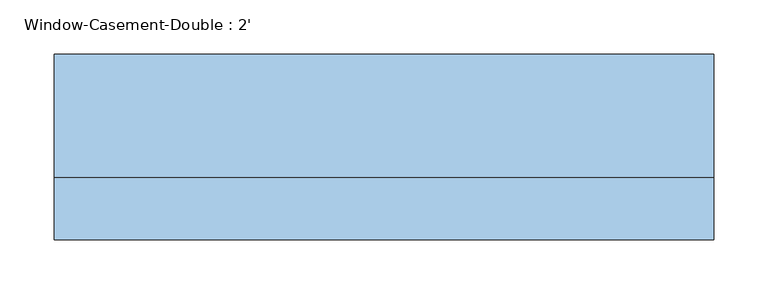
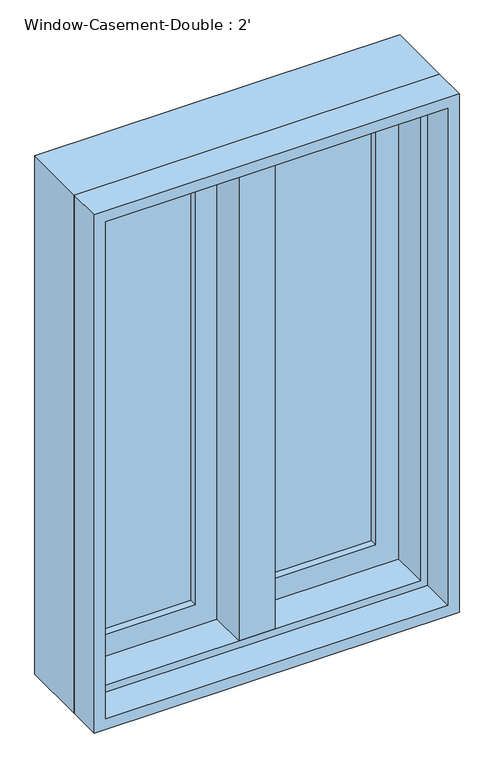
"""IFC4 building model written with IfcOpenShell, lengths in millimetres: window geometry, Window-Casement-Double : 2'."""

from ifc_helpers import new_model, si_unit, frame, origin, place, context, project, spatial, polyline, outline, extrude, faceted_brep, source, transform, mapped, element, save


def window_casement_double_2_fb285ced(model_context):
    return source(origin(), model_context, "Body", "SolidModel", [
        faceted_brep([(9.525, 95.25, 1816.1), (-9.525, 95.25, 1816.1), (-9.525, 44.45, 1816.1), (9.525, 44.45, 1816.1), (9.525, 95.25, 927.1), (9.525, 44.45, 927.1), (-9.525, 44.45, 927.1), (-9.525, 95.25, 927.1), (-9.525, 44.45, 946.15), (-9.525, 44.45, 1797.05), (-30.1625, 44.45, 946.15), (-30.1625, 44.45, 1797.05), (-30.1625, -19.05, 946.15), (-30.1625, -19.05, 1797.05), (30.1625, -19.05, 946.15), (30.1625, -19.05, 1797.05), (30.1625, 44.45, 946.15), (30.1625, 44.45, 1797.05), (9.525, 44.45, 946.15), (9.525, 44.45, 1797.05)], [[[0, 1, 2, 3]], [[4, 5, 6, 7]], [[1, 0, 4, 7]], [[2, 1, 7, 6, 8, 9]], [[9, 8, 10, 11]], [[11, 10, 12, 13]], [[13, 12, 14, 15]], [[15, 14, 16, 17]], [[17, 16, 18, 19]], [[0, 3, 19, 18, 5, 4]], [[18, 8, 6, 5]], [[9, 19, 3, 2]], [[8, 18, 16, 14, 12, 10]], [[19, 9, 11, 13, 15, 17]]]),
        extrude(outline(polyline([(-66.675, 76.2), (-66.675, 69.85), (-234.95, 69.85), (-234.95, 76.2), (-66.675, 76.2)])), frame((0.0, 0.0, 984.25), z_axis=(0.0, 0.0, 1.0), x_axis=(1.0, 0.0, 0.0)), (0.0, 0.0, 1.0), 774.7),
        extrude(outline(polyline([(-234.95, 57.15), (-234.95, 63.5), (-66.675, 63.5), (-66.675, 57.15), (-234.95, 57.15)])), frame((0.0, 0.0, 984.25), z_axis=(0.0, 0.0, 1.0), x_axis=(1.0, 0.0, 0.0)), (0.0, 0.0, 1.0), 774.7),
        extrude(outline(polyline([(234.95, 76.2), (234.95, 69.85), (66.675, 69.85), (66.675, 76.2), (234.95, 76.2)])), frame((0.0, 0.0, 984.25), z_axis=(0.0, 0.0, 1.0), x_axis=(1.0, 0.0, 0.0)), (0.0, 0.0, 1.0), 774.7),
        extrude(outline(polyline([(66.675, 57.15), (66.675, 63.5), (234.95, 63.5), (234.95, 57.15), (66.675, 57.15)])), frame((0.0, 0.0, 984.25), z_axis=(0.0, 0.0, 1.0), x_axis=(1.0, 0.0, 0.0)), (0.0, 0.0, 1.0), 774.7),
        extrude(outline(polyline([(1816.1, -292.1), (927.1, -292.1), (927.1, -9.525), (1816.1, -9.525), (1816.1, -292.1)]), holes=[polyline([(1758.95, -66.675), (984.25, -66.675), (984.25, -234.95), (1758.95, -234.95), (1758.95, -66.675)])]), frame((0.0, 44.45, 0.0), z_axis=(0.0, 1.0, 0.0), x_axis=(0.0, 0.0, 1.0)), (0.0, 0.0, 1.0), 44.45),
        extrude(outline(polyline([(927.1, 292.1), (1816.1, 292.1), (1816.1, 9.525), (927.1, 9.525), (927.1, 292.1)]), holes=[polyline([(984.25, 66.675), (1758.95, 66.675), (1758.95, 234.95), (984.25, 234.95), (984.25, 66.675)])]), frame((0.0, 44.45, 0.0), z_axis=(0.0, 1.0, 0.0), x_axis=(0.0, 0.0, 1.0)), (0.0, 0.0, 1.0), 44.45),
        extrude(outline(polyline([(1828.8, -304.8), (914.4, -304.8), (914.4, 304.8), (1828.8, 304.8), (1828.8, -304.8)]), holes=[polyline([(1809.75, 285.75), (933.45, 285.75), (933.45, -285.75), (1809.75, -285.75), (1809.75, 285.75)])]), frame((0.0, -76.2, 0.0), z_axis=(0.0, 1.0, 0.0), x_axis=(0.0, 0.0, 1.0)), (0.0, 0.0, 1.0), 57.15),
        faceted_brep([(273.05, 44.45, 1797.05), (273.05, -19.05, 1797.05), (-273.05, -19.05, 1797.05), (-273.05, 44.45, 1797.05), (292.1, 95.25, 1816.1), (292.1, 44.45, 1816.1), (-292.1, 44.45, 1816.1), (-292.1, 95.25, 1816.1), (304.8, -19.05, 1828.8), (304.8, 95.25, 1828.8), (-304.8, 95.25, 1828.8), (-304.8, -19.05, 1828.8), (-273.05, -19.05, 946.15), (-273.05, 44.45, 946.15), (-292.1, 44.45, 927.1), (-292.1, 95.25, 927.1), (-304.8, 95.25, 914.4), (-304.8, -19.05, 914.4), (273.05, -19.05, 946.15), (273.05, 44.45, 946.15), (292.1, 44.45, 927.1), (292.1, 95.25, 927.1), (304.8, 95.25, 914.4), (304.8, -19.05, 914.4)], [[[0, 1, 2, 3]], [[4, 5, 6, 7]], [[8, 9, 10, 11]], [[3, 2, 12, 13]], [[7, 6, 14, 15]], [[11, 10, 16, 17]], [[13, 12, 18, 19]], [[15, 14, 20, 21]], [[17, 16, 22, 23]], [[11, 17, 23, 8], [1, 18, 12, 2]], [[19, 18, 1, 0]], [[5, 20, 14, 6], [3, 13, 19, 0]], [[21, 20, 5, 4]], [[23, 22, 9, 8]], [[9, 22, 16, 10], [7, 15, 21, 4]]]),
    ])


if __name__ == "__main__":
    model = new_model("IFC4")
    model_context = context("Model", 3, world=origin())
    ifc_project = project(units=[si_unit("LENGTHUNIT", "METRE", prefix="MILLI")], contexts=[model_context])
    site = spatial("IfcSite", under=ifc_project)
    building = spatial("IfcBuilding", under=site)
    placement = place(None, origin())
    window_casement_double_2_shape = window_casement_double_2_fb285ced(model_context)
    element("IfcWindow", 1, ObjectType="Window-Casement-Double : 2'", at=placement, inside=building, context=model_context, shape_type="MappedRepresentation", body=[
        mapped(window_casement_double_2_shape, transform((0.0, 0.0, 0.0), x_axis=(1.0, 0.0, 0.0), y_axis=(0.0, 1.0, 0.0), z_axis=(0.0, 0.0, 1.0))),
    ])
    save(model, "model.ifc")

# Revit data of these elements
# Type "Window-Casement-Double : 2'"
#   Type Mark = "20"
#   Fire Rating = "0.5h"
#   Assembly Code = "B2020100"
#   Analytic Construction = "Double glazing - domestic"
#   Frame Extension [instance default] = 0' - 0 1/4"
#   Window Inset [instance default] = 0' - 0"
#   Wall Thickness [instance default] = 0' - 6"
#   Interior Wall Closure [instance default] = 0' - 2 1/4"
#   Half Width = 1' - 0"
#   Visual Light Transmittance = 0.81
#   Thermal Resistance (R) = 1.8146 (h·ft²·°F)/BTU
#   Solar Heat Gain Coefficient = 0.76
#   Rough Width = 2' - 0 1/2"
#   Rough Height = 3' - 0 1/2"
#   Height = 3' - 0"
#   Heat Transfer Coefficient (U) = 0.5511 BTU/(h·ft²·°F)
#   Exterior Wall Closure [instance default] = 0' - 1 1/4"
#   Extension Jamb [instance default] = 0' - 2 1/4"
#   Default Sill Height = 3' - 0"
#   Width = 2' - 0"
#   Muntin Visibility = yes
#   Interior Trim Visibility [instance default] = yes
#   Exterior Trim Visibility [instance default] = yes
#   Extension Jamb Visibility [instance default] = yes
#   Interior Trim Material = Wood - Stained
#   Muntin Pattern = Muntin Pattern_2x2 : Muntin Pattern_2x2
#   Interior Trim = Trim-Window-Interior-Flat : Picture Frame
#   Interior Frame Material = Wood - Stained
#   Glass Panel Material = Glass
#   Exterior Trim Material = Clad - White
#   Exterior Trim = Trim-Window-Exterior-Flat : with Sill
#   Exterior Frame Material = Clad - White
#   Wall Closure = (empty or 0)
# Element 1 (IfcWindow, "Window-Casement-Double : 2'")
#   Materials on its faces: "Wood - Stained", "Glass", "Clad - White"
# Materials
#   "Wood - Stained": class "Wood", colour RGB 224 178 126, transparency 0, Cost = 0
#   "Glass": class "Glass", colour RGB 0 128 192, transparency 0.75, Description = "Soda Lime Glass", Cost = 0
#   "Clad - White": class "Wood", colour RGB 242 242 238, transparency 0, Cost = 0
